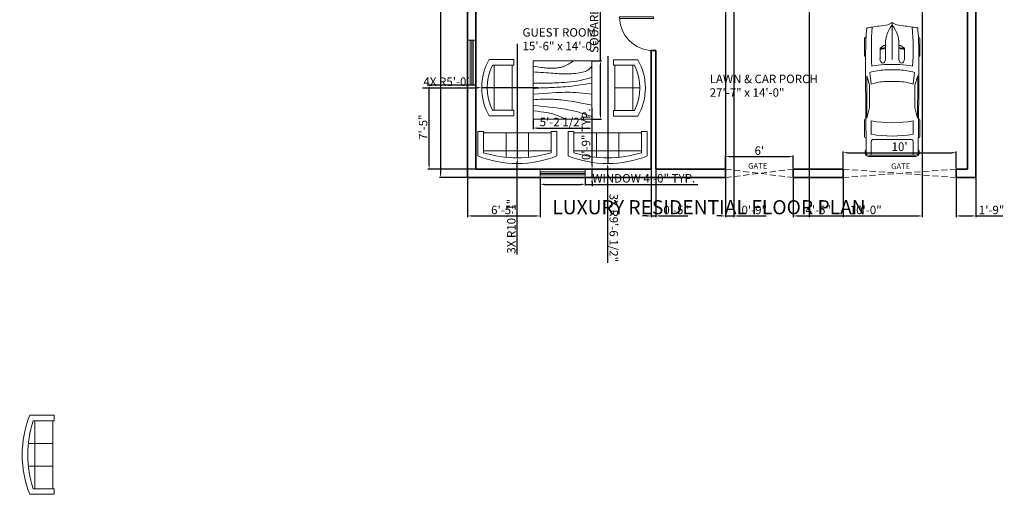
# Model space of a CAD drawing. Units: inches. Extents: x 1885 to 4781, y 1153 to 4395.
# Tile 1 of 7: x 1885 to 2931, y 1153 to 1657. Entities that reach past the tile are written whole.
import ezdxf

# ---------------------------------------------------------------- set-up
doc = ezdxf.new("R2010")
doc.units = ezdxf.units.IN
doc.linetypes.add('HIDDEN', pattern=[9.525, 6.35, -3.175])
for name, color, linetype, lineweight in [('A-ANNO-DIMS', 5, 'Continuous', 18), ('A-ANNO-TITL', 5, 'Continuous', 35), ('A-FURN', 8, 'Continuous', 18), ('A-SITE-VEHI', 8, 'Continuous', 13), ('A-WALL', 7, 'Continuous', 35)]:
    doc.layers.add(name, color=color, linetype=linetype, lineweight=lineweight)
for name, color, linetype, lineweight, true_color in [('A-ANNO-TEXT', 244, 'Continuous', 18, 0x991b1e), ('A-AREA-IDEN', 244, 'Continuous', 18, 0x991b1e), ('A-DOOR', 11, 'Continuous', 18, 0xf27172), ('A-GLAZ', 152, 'Continuous', 18, 0x2776bb), ('A-SITE-GATE', 240, 'HIDDEN', 18, 0xed1f24)]:
    doc.layers.add(name, color=color, linetype=linetype, lineweight=lineweight, true_color=true_color)
doc.styles.get("Standard").update_dxf_attribs({"font": 'arial.ttf'})
doc.dimstyles.new('ISO-25', dxfattribs={"dimtxt": 9, "dimasz": 4.5, "dimexe": 1.25, "dimexo": 0.625, "dimtad": 1, "dimdec": 0, "dimlunit": 3, "dimtxsty": 'Standard', "dimcen": 2.5, "dimadec": 0, "dimazin": 0, "dimtfac": 1, "dimtdec": 0, "dimtmove": 0, "dimatfit": 3, "dimfxl": 1, "dimarcsym": 0})

# ---------------------------------------------------------------- blocks, each defined once
blk = doc.blocks.new('Sofa - Roundback Loveseat 5 ft.')
for p, q in [((0, -32.44198), (0, -5.99998)), ((-24, -33.99998), (-24, -11.46958)), ((-23.9998, -13.38178), (23.99986, -13.38178)), ((24.00004, -33.99998), (24.00004, -11.46958)), ((-24, -32.44198), (24.00004, -32.44198))]:
    blk.add_line(p, q)
for points in [[(-24, -33.99998), (-30, -33.99998), (-30, -7.99998)], [(30.00004, -7.99998), (30.00004, -33.99998), (24.00004, -33.99998)]]:
    blk.add_lwpolyline(points)
for centre, radius, start, end in [((0, -60.24998), 60.24998, 60.13715, 119.8628), ((0, -61.38438), 55.38444, 64.32083, 115.6792)]:
    blk.add_arc(centre, radius, start, end)
blk = doc.blocks.new('Sofa - Roundback 7 ft.')
for p, q in [((-12.00002, -32.4421), (-12.00003, -6.5971)), ((11.99997, -32.4421), (11.99998, -6.5971)), ((-36.000027, -34), (-36.000027, -11.4696)), ((-35.999844, -13.3819), (35.9998, -13.3819)), ((35.99998, -34), (35.99998, -11.4696)), ((-36.000027, -32.4421), (35.99998, -32.4421))]:
    blk.add_line(p, q)
for points in [[(-36.000027, -34), (-42.000027, -34), (-42.000027, -8)], [(41.99998, -8), (41.99998, -34), (35.99998, -34)]]:
    blk.add_lwpolyline(points)
for centre, radius, start, end in [((0, -114.25), 114.25, 68.43141, 111.5686), ((-0.00001, -127.1968), 121.1968, 72.72033, 107.2797)]:
    blk.add_arc(centre, radius, start, end)
blk = doc.blocks.new('Table - Square Woodgrain 42 x 42 in.')
blk.add_line((0, -42), (42, -42))
for points in [[(0, -4), (1.704, -4.2172), (3.2358, -4.4188), (4.615, -4.604), (5.8615, -4.7721), (6.9951, -4.9224), (8.0357, -5.0541), (9.0031, -5.1667), (9.9171, -5.2594), (10.7951, -5.3316), (11.6445, -5.3836), (12.4702, -5.4157), (13.277, -5.4283), (14.0698, -5.4217), (14.8535, -5.3964), (15.6331, -5.3526), (16.4133, -5.2908), (17.1986, -5.2103), (17.9913, -5.1062), (18.793, -4.9727), (19.6056, -4.8038), (20.4307, -4.5937), (21.2701, -4.3365), (22.1256, -4.0262), (22.9989, -3.6571), (23.888, -3.2272), (24.7756, -2.7516), (25.6408, -2.2491), (26.4624, -1.7387), (27.2195, -1.2395), (27.891, -0.7703), (28.456, -0.3501), (28.8934, 0.002)], [(0, -42), (0, 0), (42, 0), (42, -42)], [(0, -8), (1.8203, -8.1001), (3.6741, -8.2149), (5.5411, -8.3408), (7.4011, -8.4741), (9.2339, -8.6112), (11.0193, -8.7484), (12.7371, -8.8821), (14.3671, -9.0086), (15.8954, -9.1246), (17.3337, -9.2278), (18.6997, -9.3159), (20.0116, -9.387), (21.2871, -9.4389), (22.5442, -9.4696), (23.8008, -9.477), (25.0749, -9.459), (26.3791, -9.4137), (27.7049, -9.3403), (29.0383, -9.2382), (30.3655, -9.1068), (31.6728, -8.9455), (32.9461, -8.7535), (34.1717, -8.5304), (35.3358, -8.2756), (36.4268, -7.9863), (37.443, -7.6521), (38.3849, -7.2603), (39.253, -6.7986), (40.048, -6.2542), (40.7705, -5.6147), (41.421, -4.8674), (42, -4)], [(42, -12), (39.1784, -12.8621), (36.4519, -13.5654), (33.8246, -14.1294), (31.3004, -14.5731), (28.8832, -14.9161), (26.577, -15.1775), (24.3858, -15.3768), (22.3136, -15.5332), (20.3622, -15.6632), (18.5254, -15.7718), (16.7947, -15.8612), (15.1618, -15.9338), (13.6183, -15.9916), (12.1558, -16.0369), (10.7659, -16.0718), (9.4403, -16.0987), (8.1703, -16.1191), (6.9461, -16.1325), (5.7577, -16.1377), (4.595, -16.1335), (3.4479, -16.1188), (2.3064, -16.0924), (1.1604, -16.0532), (0, -16)], [(42, -16), (37.6529, -16.7365), (33.8802, -17.329), (30.6179, -17.7961), (27.8015, -18.1561), (25.3668, -18.4275), (23.2497, -18.6288), (21.3859, -18.7785), (19.7111, -18.8949), (18.1693, -18.9939), (16.7375, -19.0795), (15.401, -19.1534), (14.1449, -19.217), (12.9544, -19.2717), (11.8148, -19.3191), (10.7113, -19.3606), (9.6291, -19.3976), (8.5534, -19.4323), (7.47, -19.4689), (6.3643, -19.5122), (5.222, -19.5672), (4.0288, -19.6386), (2.7703, -19.7313), (1.4321, -19.8501), (0, -20)], [(0, -24), (3.9243, -23.6805), (7.4766, -23.4138), (10.6891, -23.1954), (13.5943, -23.0205), (16.2247, -22.8847), (18.6125, -22.7832), (20.7903, -22.7116), (22.7903, -22.6651), (24.6563, -22.642), (26.4764, -22.6507), (28.35, -22.7024), (30.3766, -22.8084), (32.6555, -22.98), (35.2861, -23.2283), (38.3678, -23.5645), (42, -24)], [(42, -32), (37.392, -31.017), (33.4585, -30.2231), (30.1291, -29.5949), (27.3334, -29.109), (25.0009, -28.742), (23.0612, -28.4707), (21.4439, -28.2716), (20.0786, -28.1215), (18.8998, -28.0002), (17.8609, -27.9014), (16.9206, -27.8219), (16.0371, -27.7588), (15.1691, -27.709), (14.2748, -27.6693), (13.3128, -27.6368), (12.2415, -27.6083), (11.0295, -27.5824), (9.6867, -27.5643), (8.233, -27.5608), (6.6884, -27.5787), (5.0728, -27.6248), (3.4062, -27.7058), (1.7086, -27.8286), (0, -28)], [(0, -32), (5.4026, -32.5358), (9.9494, -33.019), (13.7424, -33.4553), (16.8834, -33.8505), (19.4743, -34.2106), (21.6171, -34.5413), (23.4136, -34.8486), (24.9657, -35.1382), (26.3614, -35.4156), (27.6332, -35.6841), (28.7995, -35.9467), (29.8788, -36.2064), (30.8897, -36.4661), (31.8507, -36.7288), (32.7802, -36.9973), (33.6968, -37.2747), (34.6175, -37.5635), (35.5531, -37.8651), (36.5128, -38.1805), (37.506, -38.5108), (38.5421, -38.8568), (39.6302, -39.2197), (40.7797, -39.6004), (42, -40)], [(0, -36), (3.0098, -36.2857), (5.5354, -36.5643), (7.6368, -36.8359), (9.374, -37.1009), (10.807, -37.3597), (11.9957, -37.6126), (13.0002, -37.8599), (13.8804, -38.102), (14.6874, -38.3393), (15.4365, -38.5729), (16.1338, -38.8041), (16.7858, -39.0341), (17.3987, -39.264), (17.9787, -39.4952), (18.5322, -39.7288), (19.0655, -39.9662), (19.5832, -40.2081), (20.0842, -40.4544), (20.5657, -40.7046), (21.0249, -40.9581), (21.459, -41.2144), (21.8653, -41.4731), (22.2409, -41.7335), (22.5831, -41.9951)]]:
    blk.add_lwpolyline(points)
blk = doc.blocks.new('*U21')
for p, q in [((536, 950), (536, 936)), ((1182, 988), (568, 988)), ((1214, 950), (1214, 950)), ((1779, 801), (2195, 746)), ((2235, 810), (1899, 912)), ((3412, 904), (3030, 807)), ((3440, 942), (3440, 950)), ((3472, 988), (4087, 988)), ((3516, 746), (3994, 746)), ((4119, 950), (4119, 934)), ((4736, 746), (4242, 746)), ((4736, -851), (4736, 851)), ((4785, -832), (4785, 832)), ((820, 295), (918, 436)), ((918, 436), (1294, 436)), ((4179, 670), (4179, -670)), ((83, 156), (3, 10)), ((756, 241), (1313, 241)), ((816, 241), (816, 283)), ((1496, -274), (1496, 274)), ((1690, -267), (1690, 267)), ((2102, 216), (2102, -216)), ((4736, -267), (4736, 267)), ((0, 0), (1313, 0)), ((3, -10), (83, -156)), ((756, -241), (1313, -241)), ((816, -241), (816, -283)), ((820, -295), (918, -436)), ((918, -436), (1294, -436)), ((536, -950), (536, -936)), ((1182, -988), (568, -988)), ((1214, -950), (1214, -950)), ((2195, -746), (1779, -801)), ((2235, -810), (1899, -912)), ((3412, -904), (3030, -807)), ((3440, -942), (3440, -950)), ((3472, -988), (4087, -988)), ((3994, -746), (3516, -746)), ((4119, -950), (4119, -934)), ((4242, -746), (4736, -746))]:
    blk.add_line(p, q)
for centre, major_axis, ratio, start_param, end_param in [((6583, -699), (0, -7755), 0.842304, 4.528606, 4.561838), ((6757, -699), (0, 7958), 0.842304, 1.367076, 1.39176), ((952, -15087), (0, -15833), 0.842304, 3.096046, 3.200911), ((1046, -12468), (0, 13417), 0.842304, 0.00281, 0.075598), ((568, 950), (0, -37.6), 0.842304, 3.141593, 4.712389), ((1638, -268113), (0, 269063), 0.842304, -0.013397, 0.002797), ((1182, 950), (0, 37.6), 0.842304, -1.570796, 0), ((3414, 137), (0, -2280), 0.842304, 4.449482, 4.652344), ((3436, 137), (0, 2077), 0.842304, 1.245306, 1.50788), ((1638, -268113), (0, -269025), 0.842304, 3.133765, 3.140441), ((3800, 71), (0, -2021), 0.842304, 4.372215, 4.640744), ((2433, -93125), (0, -93935), 0.842304, 3.134049, 3.144098), ((3472, 950), (0, -37.6), 0.842304, 3.141593, 4.712389), ((434, 0), (0, 3734), 0.842304, 4.511394, 4.913384), ((912, 0), (0, 3734), 0.842304, 4.511394, 4.913384), ((4087, 950), (0, 37.6), 0.842304, -1.570796, 0), ((4242, 670), (0, 75.2), 0.842304, 0, 1.570796), ((4588, 910), (0, 56.4), 0.842304, -0.013017, 1.249894), ((1638, -268131), (0, 269121), 0.842304, -0.013397, -0.013017), ((4673, 851), (0, -75.2), 0.842304, 1.570796, 3.128196), ((4673, 832), (0, -133), 0.842304, 1.570796, 3.128196), ((-5194, 1331), (0, -6374), 0.842304, 1.385369, 1.434372), ((331, 432), (0, 696), 0.842304, 4.435146, 4.718221), ((361, 432), (0, 696), 0.842304, 4.435146, 4.718221), ((1290, 339), (161, -9), 0.603834, -1.395552, 1.581315), ((16, 0), (0, -18.8), 0.842304, 4.131459, 5.293319), ((756, -1185), (0, 1427), 0.842304, 0, 0.590319), ((832, 283), (0, 18.8), 0.842304, 0.879714, 1.570796), ((-5194, -1331), (0, 6374), 0.842304, -1.434372, -1.385369), ((756, 1185), (0, 1427), 0.842304, 2.551274, 3.141593), ((832, -283), (0, -18.8), 0.842304, 4.712389, 5.403472), ((331, -432), (0, -696), 0.842304, 1.564964, 1.848039), ((361, -432), (0, -696), 0.842304, 1.564964, 1.848039), ((3414, -137), (0, -2280), 0.842304, -1.510751, -1.307889), ((3436, -137), (0, -2077), 0.842304, -1.50788, -1.245306), ((3800, -71), (0, -2021), 0.842304, -1.499151, -1.230623), ((6583, 699), (0, 7755), 0.842304, 1.721348, 1.754579), ((4242, -670), (0, -75.2), 0.842304, 4.712389, 6.283185), ((6757, 699), (0, 7958), 0.842304, 1.749832, 1.774517), ((952, 15087), (0, -15833), 0.842304, -0.059319, 0.045547), ((1046, 12468), (0, -13417), 0.842304, -0.075598, -0.00281), ((568, -950), (0, 37.6), 0.842304, 1.570796, 3.141593), ((1638, 268113), (0, 269063), 0.842304, 3.138796, 3.15499), ((1182, -950), (0, -37.6), 0.842304, 0, 1.570796), ((1638, 268113), (0, -269025), 0.842304, 0.001152, 0.007828), ((2433, 93125), (0, -93935), 0.842304, -0.002505, 0.007544), ((3472, -950), (0, -37.6), 0.842304, -1.570796, 0), ((4087, -950), (0, 37.6), 0.842304, 3.141593, 4.712389), ((4588, -910), (0, -56.4), 0.842304, -1.249894, 0.013017), ((1638, 268131), (0, 269121), 0.842304, 3.15461, 3.15499), ((4673, -851), (0, 75.2), 0.842304, 3.15499, 4.712389), ((4673, -832), (0, -133), 0.842304, 0.013397, 1.570796)]:
    blk.add_ellipse(centre, major_axis=major_axis, ratio=ratio, start_param=start_param, end_param=end_param)
at = {"extrusion": (0, 0, -1)}
blk.add_ellipse((1290, -339), major_axis=(161, 9), ratio=0.603834, start_param=-1.395552, end_param=1.581315, dxfattribs=at)
blk = doc.blocks.new('*D23')
at = {"layer": 'A-ANNO-DIMS', "color": 0, "lineweight": -2, "transparency": 16777216}
for p, q in [((2634.9, 1499), (2634.9, 1513)), ((2639.4, 1511.7), (2702.4, 1511.7)), ((2706.9, 1499), (2706.9, 1513))]:
    blk.add_line(p, q, dxfattribs=at)
at = {"layer": 'A-ANNO-DIMS', "color": 0, "transparency": 16777216}
for points in [[(2639.4, 1512.5), (2639.4, 1511), (2634.9, 1511.7)], [(2702.4, 1512.5), (2702.4, 1511), (2706.9, 1511.7)]]:
    blk.add_solid(points, dxfattribs=at)
at = {"layer": 'Defpoints', "color": 0, "transparency": 16777216}
for p in [(2706.9, 1511.7), (2634.9, 1498.4), (2706.9, 1498.4)]:
    blk.add_point(p, dxfattribs=at)
at = {"layer": 'A-ANNO-DIMS', "color": 0, "transparency": 16777216, "insert": (2670.9, 1516.9), "char_height": 9, "attachment_point": 5}
blk.add_mtext("6'", dxfattribs=at)
blk = doc.blocks.new('*D24')
at = {"layer": 'A-ANNO-DIMS', "color": 0, "lineweight": -2, "transparency": 16777216}
for p, q in [((2759.9, 1499), (2759.9, 1517.1)), ((2879.9, 1499), (2879.9, 1517.1)), ((2764.4, 1515.9), (2875.4, 1515.9))]:
    blk.add_line(p, q, dxfattribs=at)
at = {"layer": 'A-ANNO-DIMS', "color": 0, "transparency": 16777216}
for points in [[(2764.4, 1516.6), (2764.4, 1515.1), (2759.9, 1515.9)], [(2875.4, 1516.6), (2875.4, 1515.1), (2879.9, 1515.9)]]:
    blk.add_solid(points, dxfattribs=at)
at = {"layer": 'Defpoints', "color": 0, "transparency": 16777216}
for p in [(2879.9, 1515.9), (2759.9, 1498.4), (2879.9, 1498.4)]:
    blk.add_point(p, dxfattribs=at)
at = {"layer": 'A-ANNO-DIMS', "color": 0, "transparency": 16777216, "insert": (2819.9, 1521.1), "char_height": 9, "attachment_point": 5}
blk.add_mtext("10'", dxfattribs=at)
blk = doc.blocks.new('*D26')
at = {"layer": 'A-ANNO-DIMS', "color": 0, "lineweight": -2, "transparency": 16777216}
for p, q in [((2360.3, 2222.4), (2331, 2222.4)), ((2332.3, 2217.9), (2332.3, 1493.9)), ((2360.3, 1489.4), (2331, 1489.4))]:
    blk.add_line(p, q, dxfattribs=at)
at = {"layer": 'A-ANNO-DIMS', "color": 0, "transparency": 16777216}
for points in [[(2331.5, 2217.9), (2333, 2217.9), (2332.3, 2222.4)], [(2331.5, 1493.9), (2333, 1493.9), (2332.3, 1489.4)]]:
    blk.add_solid(points, dxfattribs=at)
at = {"layer": 'Defpoints', "color": 0, "transparency": 16777216}
for p in [(2360.9, 2222.4), (2332.3, 1489.4), (2360.9, 1489.4)]:
    blk.add_point(p, dxfattribs=at)
at = {"layer": 'A-ANNO-DIMS', "color": 0, "transparency": 16777216, "insert": (2327, 1855.9), "char_height": 9, "attachment_point": 5, "rotation": 90}
blk.add_mtext('61\'-1"', dxfattribs=at)
blk = doc.blocks.new('WIN-48IN')
for p, q in [((0, 9), (48, 9)), ((0, 0), (0, 9)), ((0, 6), (48, 6)), ((0, 4.5), (48, 4.5)), ((0, 3), (48, 3)), ((48, 9), (48, 0)), ((48, 0), (0, 0))]:
    blk.add_line(p, q)
blk = doc.blocks.new('DOOR-SWING-36IN')
for p, q in [((0, 36), (0, 0)), ((2, 36), (2, 0)), ((0, 0), (2, 0))]:
    blk.add_line(p, q)
blk.add_arc((0, 0), 36, 0, 90)
blk = doc.blocks.new('*D37')
at = {"layer": 'A-ANNO-DIMS', "color": 0, "lineweight": -2, "transparency": 16777216}
for p, q in [((2438, 1488.8), (2438, 1481)), ((2486, 1488.8), (2486, 1481)), ((2442.5, 1482.2), (2481.5, 1482.2)), ((2486, 1482.2), (2605.7, 1482.2))]:
    blk.add_line(p, q, dxfattribs=at)
at = {"layer": 'A-ANNO-DIMS', "color": 0, "transparency": 16777216}
for points in [[(2442.5, 1483), (2442.5, 1481.5), (2438, 1482.2)], [(2481.5, 1483), (2481.5, 1481.5), (2486, 1482.2)]]:
    blk.add_solid(points, dxfattribs=at)
at = {"layer": 'Defpoints', "color": 0, "transparency": 16777216}
for p in [(2438, 1489.4), (2486, 1489.4), (2486, 1482.2)]:
    blk.add_point(p, dxfattribs=at)
at = {"layer": 'A-ANNO-DIMS', "color": 0, "transparency": 16777216, "insert": (2548.1, 1487.5), "char_height": 9, "attachment_point": 5}
blk.add_mtext('WINDOW 4\'-0" TYP.', dxfattribs=at)
blk = doc.blocks.new('*D38')
at = {"layer": 'A-ANNO-DIMS', "color": 0, "lineweight": -2, "transparency": 16777216}
for p, q in [((2493.2, 1502.9), (2493.2, 1563.5)), ((2486.6, 1498.4), (2494.5, 1498.4)), ((2493.2, 1489.4), (2493.2, 1498.4)), ((2486.6, 1489.4), (2494.5, 1489.4)), ((2493.2, 1484.9), (2493.2, 1480.4))]:
    blk.add_line(p, q, dxfattribs=at)
at = {"layer": 'A-ANNO-DIMS', "color": 0, "transparency": 16777216}
for points in [[(2492.5, 1502.9), (2494, 1502.9), (2493.2, 1498.4)], [(2492.5, 1484.9), (2494, 1484.9), (2493.2, 1489.4)]]:
    blk.add_solid(points, dxfattribs=at)
at = {"layer": 'Defpoints', "color": 0, "transparency": 16777216}
for p in [(2486, 1498.4), (2493.2, 1498.4), (2486, 1489.4)]:
    blk.add_point(p, dxfattribs=at)
at = {"layer": 'A-ANNO-DIMS', "color": 0, "transparency": 16777216, "insert": (2488, 1535.5), "char_height": 9, "attachment_point": 5, "rotation": 90}
blk.add_mtext('0\'-9" TYP.', dxfattribs=at)
blk = doc.blocks.new('*D61')
at = {"layer": 'A-ANNO-DIMS', "color": 0, "lineweight": -2, "transparency": 16777216}
for p, q in [((2502.2, 1613.7), (2502.2, 1764.2)), ((2493.5, 1613.7), (2503.4, 1613.7)), ((2502.2, 1555.9), (2502.2, 1609.2)), ((2493.5, 1551.4), (2503.4, 1551.4))]:
    blk.add_line(p, q, dxfattribs=at)
at = {"layer": 'A-ANNO-DIMS', "color": 0, "transparency": 16777216}
for points in [[(2501.4, 1609.2), (2502.9, 1609.2), (2502.2, 1613.7)], [(2501.4, 1555.9), (2502.9, 1555.9), (2502.2, 1551.4)]]:
    blk.add_solid(points, dxfattribs=at)
at = {"layer": 'Defpoints', "color": 0, "transparency": 16777216}
for p in [(2492.8, 1613.7), (2502.2, 1613.7), (2492.8, 1551.4)]:
    blk.add_point(p, dxfattribs=at)
at = {"layer": 'A-ANNO-DIMS', "color": 0, "transparency": 16777216, "insert": (2496.6, 1691.2), "char_height": 9, "attachment_point": 5, "rotation": 90}
blk.add_mtext('SQUARE TABLE 5\'-2 1/2"', dxfattribs=at)
blk = doc.blocks.new('*D62')
at = {"layer": 'A-ANNO-DIMS', "color": 0, "lineweight": -2, "transparency": 16777216}
for p, q in [((2430.6, 1550.8), (2430.6, 1540.8)), ((2492.8, 1550.8), (2492.8, 1540.8)), ((2435.1, 1542.1), (2488.3, 1542.1))]:
    blk.add_line(p, q, dxfattribs=at)
at = {"layer": 'A-ANNO-DIMS', "color": 0, "transparency": 16777216}
for points in [[(2435.1, 1542.8), (2435.1, 1541.3), (2430.6, 1542.1)], [(2488.3, 1542.8), (2488.3, 1541.3), (2492.8, 1542.1)]]:
    blk.add_solid(points, dxfattribs=at)
at = {"layer": 'Defpoints', "color": 0, "transparency": 16777216}
for p in [(2430.6, 1551.4), (2492.8, 1551.4), (2492.8, 1542.1)]:
    blk.add_point(p, dxfattribs=at)
at = {"layer": 'A-ANNO-DIMS', "color": 0, "transparency": 16777216, "insert": (2461.7, 1547.4), "char_height": 9, "attachment_point": 5}
blk.add_mtext('5\'-2 1/2"', dxfattribs=at)
blk = doc.blocks.new('*D75')
at = {"layer": 'A-ANNO-DIMS', "color": 0, "lineweight": -2, "transparency": 16777216}
for p, q in [((2723.9, 1674.8), (2723.9, 1447.4)), ((2843.9, 1674.8), (2843.9, 1447.4)), ((2728.4, 1448.6), (2839.4, 1448.6))]:
    blk.add_line(p, q, dxfattribs=at)
at = {"layer": 'A-ANNO-DIMS', "color": 0, "transparency": 16777216}
for points in [[(2728.4, 1449.4), (2728.4, 1447.9), (2723.9, 1448.6)], [(2839.4, 1449.4), (2839.4, 1447.9), (2843.9, 1448.6)]]:
    blk.add_solid(points, dxfattribs=at)
at = {"layer": 'Defpoints', "color": 0, "transparency": 16777216}
for p in [(2723.9, 1675.4), (2843.9, 1675.4), (2843.9, 1448.6)]:
    blk.add_point(p, dxfattribs=at)
at = {"layer": 'A-ANNO-DIMS', "color": 0, "transparency": 16777216, "insert": (2783.9, 1453.8), "char_height": 9, "attachment_point": 5}
blk.add_mtext('10\'-0"', dxfattribs=at)
blk = doc.blocks.new('*D76')
at = {"layer": 'A-ANNO-DIMS', "color": 0, "lineweight": -2, "transparency": 16777216}
for p, q in [((2555.9, 1497.8), (2555.9, 1447.4)), ((2560.9, 1497.8), (2560.9, 1447.4)), ((2551.4, 1448.6), (2546.9, 1448.6)), ((2555.9, 1448.6), (2560.9, 1448.6)), ((2565.4, 1448.6), (2595.1, 1448.6))]:
    blk.add_line(p, q, dxfattribs=at)
at = {"layer": 'A-ANNO-DIMS', "color": 0, "transparency": 16777216}
for points in [[(2551.4, 1449.4), (2551.4, 1447.9), (2555.9, 1448.6)], [(2565.4, 1449.4), (2565.4, 1447.9), (2560.9, 1448.6)]]:
    blk.add_solid(points, dxfattribs=at)
at = {"layer": 'Defpoints', "color": 0, "transparency": 16777216}
for p in [(2555.9, 1498.4), (2560.9, 1498.4), (2560.9, 1448.6)]:
    blk.add_point(p, dxfattribs=at)
at = {"layer": 'A-ANNO-DIMS', "color": 0, "transparency": 16777216, "insert": (2582.5, 1453.8), "char_height": 9, "attachment_point": 5}
blk.add_mtext('0\'-5"', dxfattribs=at)
blk = doc.blocks.new('*D77')
at = {"layer": 'A-ANNO-DIMS', "color": 0, "lineweight": -2, "transparency": 16777216}
for p, q in [((2706.9, 1488.8), (2706.9, 1447.4)), ((2759.9, 1488.8), (2759.9, 1447.4)), ((2711.4, 1448.6), (2755.4, 1448.6))]:
    blk.add_line(p, q, dxfattribs=at)
at = {"layer": 'A-ANNO-DIMS', "color": 0, "transparency": 16777216}
for points in [[(2711.4, 1449.4), (2711.4, 1447.9), (2706.9, 1448.6)], [(2755.4, 1449.4), (2755.4, 1447.9), (2759.9, 1448.6)]]:
    blk.add_solid(points, dxfattribs=at)
at = {"layer": 'Defpoints', "color": 0, "transparency": 16777216}
for p in [(2706.9, 1489.4), (2759.9, 1489.4), (2759.9, 1448.6)]:
    blk.add_point(p, dxfattribs=at)
at = {"layer": 'A-ANNO-DIMS', "color": 0, "transparency": 16777216, "insert": (2733.4, 1453.8), "char_height": 9, "attachment_point": 5}
blk.add_mtext('4\'-5"', dxfattribs=at)
blk = doc.blocks.new('*D78')
at = {"layer": 'A-ANNO-DIMS', "color": 0, "lineweight": -2, "transparency": 16777216}
for p, q in [((2879.9, 1488.8), (2879.9, 1447.4)), ((2900.9, 1488.8), (2900.9, 1447.4)), ((2884.4, 1448.6), (2896.4, 1448.6)), ((2900.9, 1448.6), (2929.7, 1448.6))]:
    blk.add_line(p, q, dxfattribs=at)
at = {"layer": 'A-ANNO-DIMS', "color": 0, "transparency": 16777216}
for points in [[(2884.4, 1449.4), (2884.4, 1447.9), (2879.9, 1448.6)], [(2896.4, 1449.4), (2896.4, 1447.9), (2900.9, 1448.6)]]:
    blk.add_solid(points, dxfattribs=at)
at = {"layer": 'Defpoints', "color": 0, "transparency": 16777216}
for p in [(2879.9, 1489.4), (2900.9, 1489.4), (2900.9, 1448.6)]:
    blk.add_point(p, dxfattribs=at)
at = {"layer": 'A-ANNO-DIMS', "color": 0, "transparency": 16777216, "insert": (2917.6, 1453.8), "char_height": 9, "attachment_point": 5}
blk.add_mtext('1\'-9"', dxfattribs=at)
blk = doc.blocks.new('*D82')
at = {"layer": 'A-ANNO-DIMS', "color": 0, "lineweight": -2, "transparency": 16777216}
for p, q in [((2360.9, 1488.8), (2360.9, 1447.4)), ((2438, 1488.8), (2438, 1447.4)), ((2365.4, 1448.6), (2433.5, 1448.6))]:
    blk.add_line(p, q, dxfattribs=at)
at = {"layer": 'A-ANNO-DIMS', "color": 0, "transparency": 16777216}
for points in [[(2365.4, 1449.4), (2365.4, 1447.9), (2360.9, 1448.6)], [(2433.5, 1449.4), (2433.5, 1447.9), (2438, 1448.6)]]:
    blk.add_solid(points, dxfattribs=at)
at = {"layer": 'Defpoints', "color": 0, "transparency": 16777216}
for p in [(2360.9, 1489.4), (2438, 1489.4), (2438, 1448.6)]:
    blk.add_point(p, dxfattribs=at)
at = {"layer": 'A-ANNO-DIMS', "color": 0, "transparency": 16777216, "insert": (2399.5, 1453.8), "char_height": 9, "attachment_point": 5}
blk.add_mtext('6\'-5"', dxfattribs=at)
blk = doc.blocks.new('*D83')
at = {"layer": 'A-ANNO-DIMS', "color": 0, "lineweight": -2, "transparency": 16777216}
for p, q in [((2369.3, 1587.7), (2318.9, 1587.7)), ((2320.1, 1502.9), (2320.1, 1583.2)), ((2369.3, 1498.4), (2318.9, 1498.4))]:
    blk.add_line(p, q, dxfattribs=at)
at = {"layer": 'A-ANNO-DIMS', "color": 0, "transparency": 16777216}
for points in [[(2319.4, 1583.2), (2320.9, 1583.2), (2320.1, 1587.7)], [(2319.4, 1502.9), (2320.9, 1502.9), (2320.1, 1498.4)]]:
    blk.add_solid(points, dxfattribs=at)
at = {"layer": 'Defpoints', "color": 0, "transparency": 16777216}
for p in [(2320.1, 1587.7), (2369.9, 1587.7), (2369.9, 1498.4)]:
    blk.add_point(p, dxfattribs=at)
at = {"layer": 'A-ANNO-DIMS', "color": 0, "transparency": 16777216, "insert": (2314.9, 1543), "char_height": 9, "attachment_point": 5, "rotation": 90}
blk.add_mtext('7\'-5"', dxfattribs=at)
blk = doc.blocks.new('*D91')
at = {"layer": 'A-ANNO-DIMS', "color": 0, "lineweight": -2, "transparency": 16777216}
for p, q in [((2634.9, 1674.8), (2634.9, 1447.4)), ((2643.9, 1674.8), (2643.9, 1447.4)), ((2630.4, 1448.6), (2625.9, 1448.6)), ((2634.9, 1448.6), (2643.9, 1448.6)), ((2648.4, 1448.6), (2678.1, 1448.6))]:
    blk.add_line(p, q, dxfattribs=at)
at = {"layer": 'A-ANNO-DIMS', "color": 0, "transparency": 16777216}
for points in [[(2630.4, 1449.4), (2630.4, 1447.9), (2634.9, 1448.6)], [(2648.4, 1449.4), (2648.4, 1447.9), (2643.9, 1448.6)]]:
    blk.add_solid(points, dxfattribs=at)
at = {"layer": 'Defpoints', "color": 0, "transparency": 16777216}
for p in [(2634.9, 1675.4), (2643.9, 1675.4), (2643.9, 1448.6)]:
    blk.add_point(p, dxfattribs=at)
at = {"layer": 'A-ANNO-DIMS', "color": 0, "transparency": 16777216, "insert": (2665.5, 1453.8), "char_height": 9, "attachment_point": 5}
blk.add_mtext('0\'-9"', dxfattribs=at)
blk = doc.blocks.new('*D93')
at = {"layer": 'A-ANNO-DIMS', "color": 0, "lineweight": -2, "transparency": 16777216}
for p, q in [((2413.8, 1631.6), (2413.8, 1510.4)), ((2413.8, 1407.6), (2413.8, 1505.9))]:
    blk.add_line(p, q, dxfattribs=at)
at = {"layer": 'A-ANNO-DIMS', "color": 0, "transparency": 16777216}
blk.add_solid([(2413.1, 1505.9), (2414.6, 1505.9), (2413.8, 1510.4)], dxfattribs=at)
at = {"layer": 'Defpoints', "color": 0, "transparency": 16777216}
for p in [(2413.8, 1631.6), (2413.8, 1510.4)]:
    blk.add_point(p, dxfattribs=at)
at = {"layer": 'A-ANNO-DIMS', "color": 0, "transparency": 16777216, "insert": (2408.6, 1437.7), "char_height": 9, "attachment_point": 5, "rotation": 90}
blk.add_mtext('3X R10\'-1"', dxfattribs=at)
blk = doc.blocks.new('*D94')
at = {"layer": 'A-ANNO-DIMS', "color": 0, "lineweight": -2, "transparency": 16777216}
for p, q in [((2509.8, 1618.7), (2509.8, 1504.4)), ((2509.8, 1398.8), (2509.8, 1499.9))]:
    blk.add_line(p, q, dxfattribs=at)
at = {"layer": 'A-ANNO-DIMS', "color": 0, "transparency": 16777216}
blk.add_solid([(2510.6, 1499.9), (2509.1, 1499.9), (2509.8, 1504.4)], dxfattribs=at)
at = {"layer": 'Defpoints', "color": 0, "transparency": 16777216}
for p in [(2509.8, 1618.7), (2509.8, 1504.4)]:
    blk.add_point(p, dxfattribs=at)
at = {"layer": 'A-ANNO-DIMS', "color": 0, "transparency": 16777216, "insert": (2515.1, 1435.9), "char_height": 9, "attachment_point": 5, "rotation": 270.0001}
blk.add_mtext('3X R9\'-6 1/2"', dxfattribs=at)
blk = doc.blocks.new('*D95')
at = {"layer": 'A-ANNO-DIMS', "color": 0, "lineweight": -2, "transparency": 16777216}
for p, q in [((2313.1, 1585), (2371.4, 1585)), ((2436.2, 1585), (2375.9, 1585))]:
    blk.add_line(p, q, dxfattribs=at)
at = {"layer": 'A-ANNO-DIMS', "color": 0, "transparency": 16777216}
blk.add_solid([(2371.4, 1585.8), (2371.4, 1584.3), (2375.9, 1585)], dxfattribs=at)
at = {"layer": 'Defpoints', "color": 0, "transparency": 16777216}
for p in [(2375.9, 1585), (2436.2, 1585)]:
    blk.add_point(p, dxfattribs=at)
at = {"layer": 'A-ANNO-DIMS', "color": 0, "transparency": 16777216, "insert": (2339.8, 1590.2), "char_height": 9, "attachment_point": 5, "rotation": 359.9996}
blk.add_mtext('4X R5\'-0"', dxfattribs=at)

msp = doc.modelspace()

# ---------------------------------------------------------------- linework, layer by layer
at = {"layer": 'A-SITE-GATE'}
for p, q in [((2634.91, 1498.42), (2706.91, 1489.42)), ((2634.91, 1489.42), (2706.91, 1498.42)), ((2759.91, 1498.42), (2879.91, 1489.42)), ((2879.91, 1498.42), (2759.91, 1489.42))]:
    msp.add_line(p, q, dxfattribs=at)
at = {"layer": 'A-WALL'}
for p, q in [((2360.91, 2222.42), (2360.91, 1489.42)), ((2900.91, 2222.42), (2900.91, 1489.42)), ((2369.91, 1666.42), (2369.91, 1498.42)), ((2891.91, 1666.42), (2891.91, 1498.42)), ((2555.91, 1624.42), (2560.91, 1624.42)), ((2555.91, 1624.42), (2555.91, 1498.42)), ((2560.91, 1624.42), (2560.91, 1498.42)), ((2369.91, 1498.42), (2555.91, 1498.42)), ((2560.91, 1498.42), (2634.91, 1498.42)), ((2634.91, 1489.42), (2634.91, 1498.42)), ((2706.91, 1489.42), (2706.91, 1498.42)), ((2706.91, 1498.42), (2759.91, 1498.42)), ((2759.91, 1498.42), (2759.91, 1489.42)), ((2879.91, 1498.42), (2879.91, 1489.42)), ((2879.91, 1498.42), (2891.91, 1498.42)), ((2360.91, 1489.42), (2634.91, 1489.42)), ((2706.91, 1489.42), (2759.91, 1489.42)), ((2879.91, 1489.42), (2900.91, 1489.42))]:
    msp.add_line(p, q, dxfattribs=at)

# ---------------------------------------------------------------- block references
at = {"layer": 'A-DOOR', "extrusion": (0, 0, -1), "zscale": -1, "rotation": 269.9999999999985}
msp.add_blockref('DOOR-SWING-36IN', (-2558.41, 1660.42), dxfattribs=at)
at = {"layer": 'A-FURN'}
for name, p, rotation in [('Sofa - Roundback Loveseat 5 ft.', (2375.95, 1585.01), 89.99999999999999), ('Sofa - Roundback Loveseat 5 ft.', (2549.91, 1584.78), 270), ('Sofa - Roundback 7 ft.', (2413.8, 1504.42), 180), ('Sofa - Roundback 7 ft.', (2509.83, 1504.4), 180), ('Sofa - Roundback 7 ft.', (1887.88, 1194.63), 89.99999999999991)]:
    msp.add_blockref(name, p, dxfattribs=dict(at, rotation=rotation))
at = {"layer": 'A-FURN', "xscale": 1.482526926039659, "yscale": 1.482526926039659, "zscale": 1.482526926039659}
msp.add_blockref('Table - Square Woodgrain 42 x 42 in.', (2430.58, 1613.69), dxfattribs=at)
at = {"layer": 'A-GLAZ', "rotation": 90.00000000000328}
msp.add_blockref('WIN-48IN', (2369.91, 1587.67), dxfattribs=at)
at = {"layer": 'A-GLAZ'}
msp.add_blockref('WIN-48IN', (2438.02, 1489.42), dxfattribs=at)
at = {"layer": 'A-SITE-VEHI', "xscale": 0.0297448494413493, "yscale": 0.0297448494413493, "zscale": 0.0297448494413493, "rotation": 270}
msp.add_blockref('*U21', (2812.06, 1654.21), dxfattribs=at)

# ---------------------------------------------------------------- texts
at = {"layer": 'A-ANNO-TEXT'}
for p in [(2659.04, 1498.89), (2810.95, 1498.42)]:
    msp.add_text('GATE', height=6, dxfattribs=at).set_placement(p)
at = {"layer": 'A-ANNO-TITL'}
msp.add_text('LUXURY RESIDENTIAL FLOOR PLAN', height=15, dxfattribs=at).set_placement((2450.95, 1450.42))
at = {"layer": 'A-AREA-IDEN'}
for s, p in [('GUEST ROOM', (2419.35, 1639.26)), ('15\'-6" x 14\'-0"', (2419.35, 1624.8)), ('LAWN & CAR PORCH', (2618.15, 1589.82)), ('27\'-7" x 14\'-0"', (2618.15, 1575.36))]:
    msp.add_text(s, height=9, dxfattribs=at).set_placement(p)

# ---------------------------------------------------------------- dimensions: what is measured, and where the dimension line sits
at = {"layer": 'A-ANNO-DIMS'}
for base, p1, p2, override, picture, middle in [((2332.27, 1489.42), (2360.91, 2222.42), (2360.91, 1489.42), {"dimclrd": 0, "dimclre": 0, "dimclrt": 0}, '*D26', (2327.04, 1855.92)), ((2320.1075, 1587.6681), (2369.9075, 1498.421), (2369.9075, 1587.6681), {"dimdec": 1, "dimlfac": 1, "dimrnd": 0, "dimzin": 1, "dimdsep": 46, "dimlunit": 4, "dimfrac": 2}, '*D83', (2314.9058, 1543.0446))]:
    dim = msp.add_linear_dim(base=base, p1=p1, p2=p2, angle=90, dimstyle='ISO-25', override=override, dxfattribs=at)
    dim.commit()
    dim.dimension.update_dxf_attribs({"geometry": picture, "text_midpoint": middle})
for base, p1, p2, text, picture, middle in [((2502.19, 1613.69), (2492.84, 1551.42), (2492.84, 1613.69), 'SQUARE TABLE <>', '*D61', (2496.63, 1691.2)), ((2493.22, 1498.42), (2486.02, 1489.42), (2486.02, 1498.42), '<> TYP.', '*D38', (2488, 1535.48))]:
    dim = msp.add_linear_dim(base=base, p1=p1, p2=p2, angle=90, text=text, dimstyle='ISO-25', override={"dimdec": 1, "dimlfac": 1, "dimrnd": 0, "dimzin": 1, "dimdsep": 46, "dimlunit": 4, "dimfrac": 2}, dxfattribs=at)
    dim.commit()
    dim.dimension.update_dxf_attribs({"geometry": picture, "text_midpoint": middle})
for base, p1, p2, override, picture, middle in [((2643.91, 1448.62), (2634.91, 1675.42), (2643.91, 1675.42), {"dimdec": 1, "dimlfac": 1, "dimrnd": 0, "dimzin": 1, "dimdsep": 46, "dimlunit": 4, "dimfrac": 2}, '*D91', (2665.49, 1453.84)), ((2843.91, 1448.62), (2723.91, 1675.42), (2843.91, 1675.42), {"dimdec": 1, "dimlfac": 1, "dimrnd": 0, "dimzin": 1, "dimdsep": 46, "dimlunit": 4, "dimfrac": 2}, '*D75', (2783.91, 1453.84)), ((2492.84, 1542.08), (2430.58, 1551.42), (2492.84, 1551.42), {"dimdec": 1, "dimlfac": 1, "dimrnd": 0, "dimzin": 1, "dimdsep": 46, "dimlunit": 4, "dimfrac": 2}, '*D62', (2461.71, 1547.36)), ((2879.91, 1515.85), (2759.91, 1498.42), (2879.91, 1498.42), {"dimclrd": 0, "dimclre": 0, "dimclrt": 0}, '*D24', (2819.91, 1521.07)), ((2706.91, 1511.73), (2634.91, 1498.42), (2706.91, 1498.42), {"dimclrd": 0, "dimclre": 0, "dimclrt": 0}, '*D23', (2670.91, 1516.95)), ((2560.91, 1448.62), (2555.91, 1498.42), (2560.91, 1498.42), {"dimdec": 1, "dimlfac": 1, "dimrnd": 0, "dimzin": 1, "dimdsep": 46, "dimlunit": 4, "dimfrac": 2}, '*D76', (2582.49, 1453.84)), ((2438.02, 1448.62), (2360.91, 1489.42), (2438.02, 1489.42), {"dimdec": 1, "dimlfac": 1, "dimrnd": 0, "dimzin": 1, "dimdsep": 46, "dimlunit": 4, "dimfrac": 2}, '*D82', (2399.46, 1453.84)), ((2759.91, 1448.62), (2706.91, 1489.42), (2759.91, 1489.42), {"dimdec": 1, "dimlfac": 1, "dimrnd": 0, "dimzin": 1, "dimdsep": 46, "dimlunit": 4, "dimfrac": 2}, '*D77', (2733.41, 1453.82)), ((2900.91, 1448.62), (2879.91, 1489.42), (2900.91, 1489.42), {"dimdec": 1, "dimlfac": 1, "dimrnd": 0, "dimzin": 1, "dimdsep": 46, "dimlunit": 4, "dimfrac": 2}, '*D78', (2917.57, 1453.84))]:
    dim = msp.add_linear_dim(base=base, p1=p1, p2=p2, dimstyle='ISO-25', override=override, dxfattribs=at)
    dim.commit()
    dim.dimension.update_dxf_attribs({"geometry": picture, "text_midpoint": middle})
for center, mpoint, text, picture, middle in [((2413.8, 1631.61), (2413.8, 1510.42), '3X <>', '*D93', (2413.8, 1437.7)), ((2509.83, 1618.65), (2509.84, 1504.4), '3X <>', '*D94', (2509.84, 1435.85)), ((2436.19827, 1585.01157), (2375.94829, 1585.012), '4X <>', '*D95', (2339.7983, 1585.01226))]:
    dim = msp.add_radius_dim(center=center, mpoint=mpoint, text=text, dimstyle='ISO-25', override={"dimdec": 1, "dimlfac": 1, "dimrnd": 0, "dimzin": 1, "dimdsep": 46, "dimlunit": 4, "dimfrac": 2}, dxfattribs=at)
    dim.commit()
    dim.dimension.update_dxf_attribs({"geometry": picture, "text_midpoint": middle, "dimtype": 164})
dim = msp.add_linear_dim(base=(2486.02, 1482.22), p1=(2438.02, 1489.42), p2=(2486.02, 1489.42), text='WINDOW <> TYP.', dimstyle='ISO-25', override={"dimdec": 1, "dimlfac": 1, "dimrnd": 0, "dimzin": 1, "dimdsep": 46, "dimlunit": 4, "dimfrac": 2}, dxfattribs=at)
dim.commit()
dim.dimension.update_dxf_attribs({"geometry": '*D37', "text_midpoint": (2548.09, 1487.5)})

doc.saveas('drawing.dxf')
